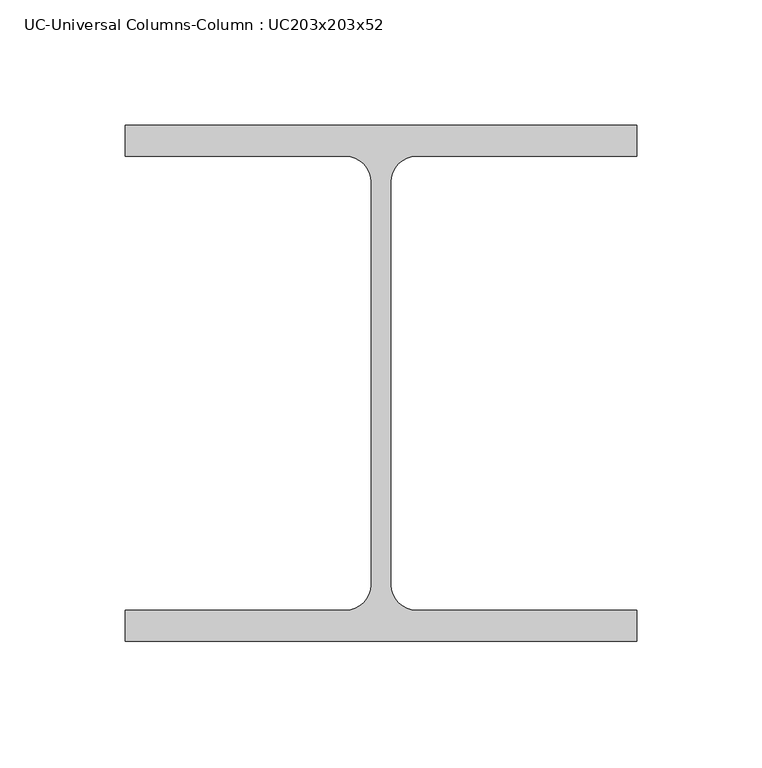
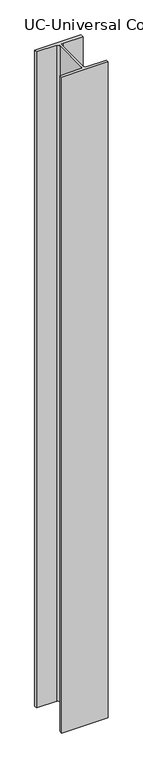
"""IFC4 building model written with IfcOpenShell, lengths in millimetres: column geometry, UC-Universal Columns-Column : UC203x203x52."""

from ifc_helpers import new_model, si_unit, point, frame_2d, origin, origin_with_axes, place, context, project, spatial, polyline, circle_curve, trimmed, segment, composite_curve, outline, extrude, source, transform, mapped, element, save


def uc_universal_columns_column_uc203x203x52_f24fe326(model_context):
    return source(origin(), model_context, "Body", "SweptSolid", [
        extrude(outline(composite_curve([segment(polyline([(102.15, 103.1), (102.15, 90.6), (14.15, 90.6)]), True, "CONTINUOUS"), segment(trimmed(circle_curve(frame_2d((14.15, 80.4)), 10.2), [point((14.15, 90.6))], [point((3.95, 80.4))], True, "CARTESIAN"), True, "CONTINUOUS"), segment(polyline([(3.95, 80.4), (3.95, -80.4)]), True, "CONTINUOUS"), segment(trimmed(circle_curve(frame_2d((14.15, -80.4)), 10.2), [point((3.95, -80.4))], [point((14.15, -90.6))], True, "CARTESIAN"), True, "CONTINUOUS"), segment(polyline([(14.15, -90.6), (102.15, -90.6), (102.15, -103.1), (-102.15, -103.1), (-102.15, -90.6), (-14.15, -90.6)]), True, "CONTINUOUS"), segment(trimmed(circle_curve(frame_2d((-14.15, -80.4)), 10.2), [point((-14.15, -90.6))], [point((-3.95, -80.4))], True, "CARTESIAN"), True, "CONTINUOUS"), segment(polyline([(-3.95, -80.4), (-3.95, 80.4)]), True, "CONTINUOUS"), segment(trimmed(circle_curve(frame_2d((-14.15, 80.4)), 10.2), [point((-3.95, 80.4))], [point((-14.15, 90.6))], True, "CARTESIAN"), True, "CONTINUOUS"), segment(polyline([(-14.15, 90.6), (-102.15, 90.6), (-102.15, 103.1), (102.15, 103.1)]), True, "CONTINUOUS")], self_intersect=False)), origin_with_axes(), (0.0, 0.0, 1.0), 3048.0),
    ])


if __name__ == "__main__":
    model = new_model("IFC4")
    model_context = context("Model", 3, world=origin())
    ifc_project = project(units=[si_unit("LENGTHUNIT", "METRE", prefix="MILLI")], contexts=[model_context])
    site = spatial("IfcSite", under=ifc_project)
    building = spatial("IfcBuilding", under=site)
    placement = place(None, origin())
    uc_universal_columns_column_uc203x203x52_shape = uc_universal_columns_column_uc203x203x52_f24fe326(model_context)
    element("IfcColumn", 1, ObjectType="UC-Universal Columns-Column : UC203x203x52", at=placement, inside=building, context=model_context, shape_type="MappedRepresentation", body=[
        mapped(uc_universal_columns_column_uc203x203x52_shape, transform((0.0, 0.0, 0.0), x_axis=(1.0, 0.0, 0.0), y_axis=(0.0, 1.0, 0.0), z_axis=(0.0, 0.0, 1.0))),
    ])
    save(model, "model.ifc")

# Revit data of these elements
# Type "UC-Universal Columns-Column : UC203x203x52"
#   Section Name Key = "UC203x203x52"
#   Width = 20.43 cm
#   Web Thickness = 0.79 cm
#   Web Fillet = 1.02 cm
#   Warping Constant = 167000.0 cm⁶
#   Torsional Moment of Inertia = 31.80 cm⁴
#   Section Area = 66.0 cm²
#   Plastic Modulus weak axis = 264.0 cm³
#   Plastic Modulus strong axis = 567.0 cm³
#   Nominal Weight = 51.9998 kgf/m
#   Moment of Inertia weak axis = 1778.00 cm⁴
#   Moment of Inertia strong axis = 5259.00 cm⁴
#   Height = 20.62 cm
#   Flange Thickness = 1.25 cm
#   Elastic Modulus weak axis = 174.0 cm³
#   Elastic Modulus strong axis = 510.0 cm³
#   Centroid Vertical = 10.31 cm
#   Centroid Horizontal = 10.215 cm
#   Bolt Spacing = 14.0 cm
#   Structural Material [instance default] = Metal - Steel 43-275
#   Type Comments = ""
#   Assembly Code = ""
# Element 1 (IfcColumn, "UC-Universal Columns-Column : UC203x203x52")
#   Materials on its faces: "Metal - Steel 43-275"
# Materials
#   "Metal - Steel 43-275": class "Metal", colour RGB 247 247 247, transparency 0, Cost = 0
